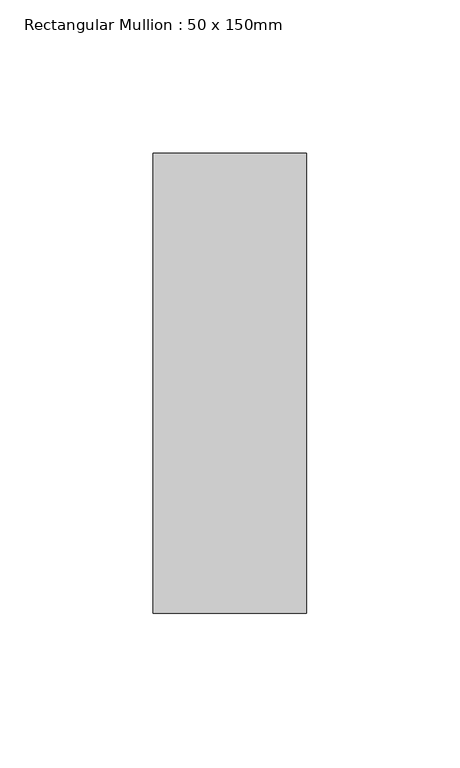
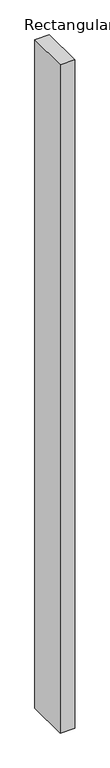
"""IFC4 building model written with IfcOpenShell, lengths in millimetres: member geometry, Rectangular Mullion : 50 x 150mm."""

from ifc_helpers import new_model, si_unit, frame, origin, place, context, project, spatial, polyline, outline, extrude, source, transform, mapped, element, save


def rectangular_mullion_50_x_150mm_c59a77fc(model_context):
    return source(origin(), model_context, "Body", "SweptSolid", [
        extrude(outline(polyline([(25.0, 75.0), (25.0, -75.0), (-25.0, -75.0), (-25.0, 75.0), (25.0, 75.0)])), frame((0.0, 0.0, -2425.0), z_axis=(0.0, 0.0, 1.0), x_axis=(1.0, 0.0, 0.0)), (0.0, 0.0, 1.0), 2425.0),
    ])


if __name__ == "__main__":
    model = new_model("IFC4")
    model_context = context("Model", 3, world=origin())
    ifc_project = project(units=[si_unit("LENGTHUNIT", "METRE", prefix="MILLI")], contexts=[model_context])
    site = spatial("IfcSite", under=ifc_project)
    building = spatial("IfcBuilding", under=site)
    placement = place(None, origin())
    rectangular_mullion_50_x_150mm_shape = rectangular_mullion_50_x_150mm_c59a77fc(model_context)
    element("IfcMember", 1, ObjectType="Rectangular Mullion : 50 x 150mm", at=placement, inside=building, context=model_context, shape_type="MappedRepresentation", body=[
        mapped(rectangular_mullion_50_x_150mm_shape, transform((0.0, 0.0, 0.0), x_axis=(1.0, 0.0, 0.0), y_axis=(0.0, 1.0, 0.0), z_axis=(0.0, 0.0, 1.0))),
    ])
    save(model, "model.ifc")

# Revit data of these elements
# Type "Rectangular Mullion : 50 x 150mm"
#   built-in parameter 1007304 = 0.492126 (stored number, unit not read)
#   built-in parameter 1007301 = 0.082021 (stored number, unit not read)
#   built-in parameter 1007300 = 0.082021 (stored number, unit not read)
# Element 1 (IfcMember, "Rectangular Mullion : 50 x 150mm")
#   Materials on its faces: "Aluminium"
# Materials
#   "Aluminium": class "Metal", colour RGB 247 247 247, transparency 0, Description = "Aluminium 6061", Cost = 0
